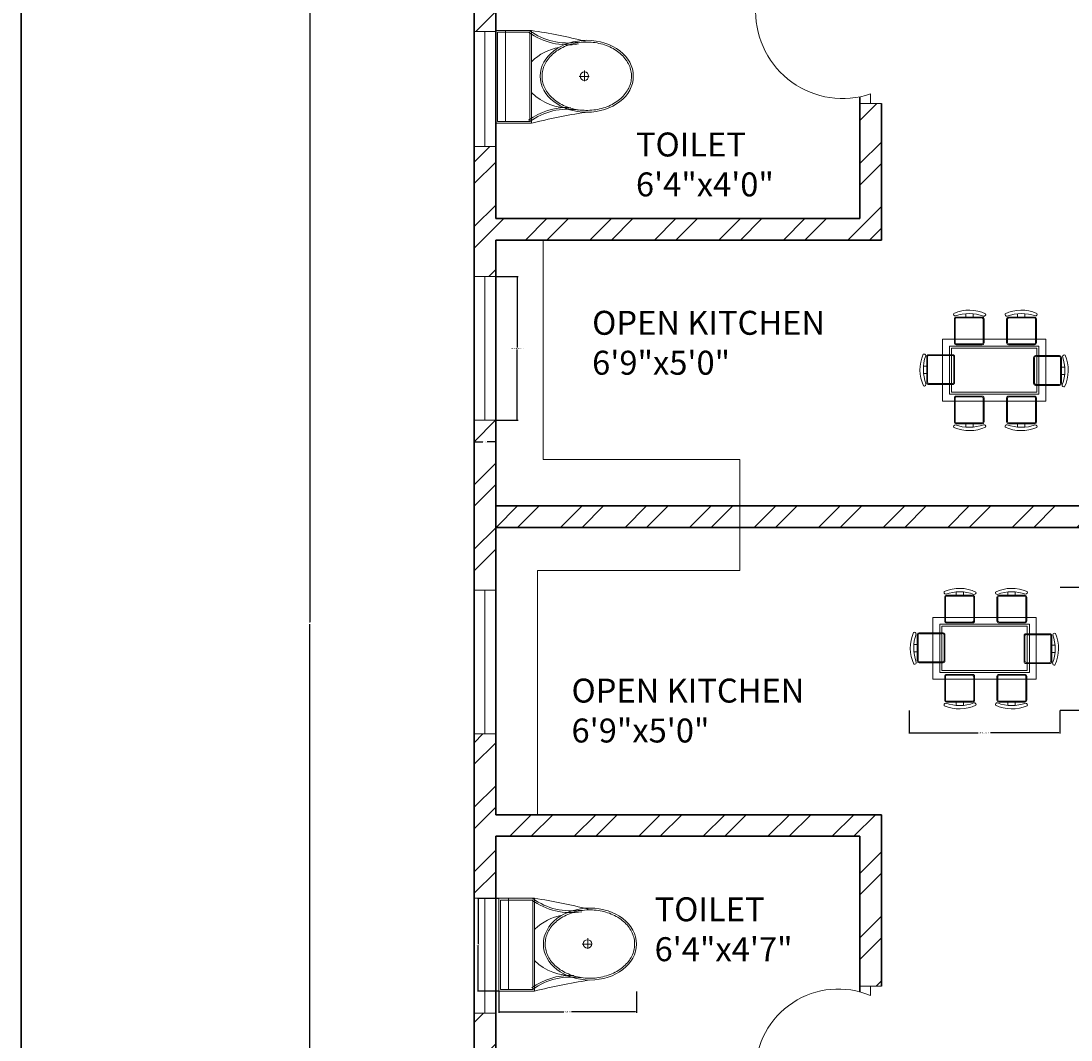
# Model space of a CAD drawing. Units: inches. Extents: x 2165 to 3042, y 1626 to 2968.
# Tile 2 of 11: x 2192 to 2411, y 1996 to 2208. Entities that reach past the tile are written whole.
import ezdxf

# ---------------------------------------------------------------- set-up
doc = ezdxf.new("R2010")
doc.units = ezdxf.units.IN
for name, color, linetype, lineweight in [('A-ANNO-DIMS', 2, 'Continuous', 18), ('A-AREA-IDEN', 7, 'Continuous', 18), ('A-DOOR', 3, 'Continuous', 18), ('A-FLOR-CASE', 8, 'Continuous', 18), ('A-FLOR-FIXT', 9, 'Continuous', 18), ('A-FURN', 8, 'Continuous', 13), ('A-GLAZ', 4, 'Continuous', 18), ('A-WALL', 7, 'Continuous', 35), ('A-WALL-PATT', 252, 'Continuous', 13)]:
    doc.layers.add(name, color=color, linetype=linetype, lineweight=lineweight)
doc.styles.get("Standard").update_dxf_attribs({"font": 'arial.ttf'})
doc.dimstyles.get("Standard").update_dxf_attribs({"dimtxt": 0.18, "dimasz": 0.18, "dimexe": 0.18, "dimexo": 0.0625, "dimgap": 0.09, "dimtad": 0, "dimtih": 1, "dimtoh": 1, "dimdec": 4, "dimzin": 0, "dimdsep": 46, "dimtxsty": 'Standard', "dimcen": 0.09, "dimadec": 0, "dimazin": 0, "dimtfac": 1, "dimtdec": 4, "dimtofl": 0, "dimtmove": 0, "dimatfit": 3, "dimfxl": 1, "dimtolj": 1, "dimtzin": 0, "dimarcsym": 0})

# ---------------------------------------------------------------- blocks, each defined once
blk = doc.blocks.new('A$C31115884')
for p, q in [((283.1, 497.7), (223.4, 497.7)), ((257.5, 466.4), (257.5, 523.2)), ((0, 200), (0, 0)), ((520, 200), (0, 200)), ((10, 190), (10, 10)), ((510, 190), (10, 190)), ((510, 10), (510, 190)), ((520, 0), (520, 200)), ((510, 54.5), (0, 54.5)), ((10, 10), (510, 10)), ((0, 0), (520, 0))]:
    blk.add_line(p, q)
blk.add_circle((255.6, 496.4), 23.6)
for centre, radius, start, end in [((2777.7, -204.6), 2807, 165.4549, 171.71327), ((3237, 905), 2807, 188.28673, 194.5451), ((-294.5, 403.3), 364.7, 324.20913, 9.34987), ((-294.5, 403.3), 374.7, 324.20913, 9.34987), ((139.5, 406.2), 293.5, 315.84364, 2.65635), ((805.8, 403.3), 364.7, 170.65013, 215.79087), ((383.6, 406.2), 293.5, 190.27735, 224.15636), ((805.8, 403.3), 374.7, 179.20365, 215.79087)]:
    blk.add_arc(centre, radius, start, end)
blk.add_ellipse((256.2, 509.9), major_axis=(0, -260.7), ratio=0.772727)
blk.add_open_spline([(256.2, 259.2), (263.1, 259.2), (270, 259.7), (287.8, 262.3), (298.7, 265.1), (319.9, 273.1), (330.2, 278.4), (350.1, 291.1), (359.7, 298.7), (377.7, 315.9), (386.2, 325.5), (401.7, 346.6), (408.8, 358.1), (421.3, 382.5), (426.8, 395.5), (435.9, 422.4), (439.5, 436.4), (444.8, 465.1), (446.5, 479.7), (447.9, 509.2), (447.6, 524), (445, 553.3), (442.7, 567.8), (436.3, 596), (432.1, 609.7), (421.9, 636), (416, 648.6), (402.5, 672.1), (395, 683), (378.6, 703), (369.8, 712.1), (351.1, 728), (341.3, 734.8), (320.9, 746.2), (310.4, 750.7), (288.9, 757.3), (278, 759.4), (256, 761), (245, 760.6), (223.1, 757.2), (212.3, 754.3), (191.1, 746.1), (180.8, 740.7), (160.9, 727.8), (151.4, 720.1), (133.5, 702.7), (125.1, 693), (109.6, 671.7), (102.6, 660.2), (90.2, 635.7), (84.9, 622.7), (76, 595.6), (72.4, 581.6), (67.2, 552.9), (65.6, 538.2), (64.4, 508.8), (64.8, 494), (67.5, 464.7), (69.9, 450.2), (76.6, 422), (80.8, 408.3), (91.1, 382.2), (97.2, 369.7), (110.8, 346.3), (118.4, 335.4), (134.8, 315.6), (143.7, 306.7), (162.4, 290.9), (172.3, 284.2), (192.8, 273), (203.3, 268.6), (224.8, 262.2), (235.8, 260.2), (249.9, 259.3), (253, 259.2), (256.2, 259.2)], degree=3, knots=[0, 0, 0, 0, 0.110105, 0.110105, 0.285049, 0.285049, 0.459994, 0.459994, 0.634938, 0.634938, 0.809882, 0.809882, 0.984827, 0.984827, 1.159771, 1.159771, 1.334715, 1.334715, 1.50966, 1.50966, 1.684604, 1.684604, 1.859549, 1.859549, 2.034493, 2.034493, 2.209437, 2.209437, 2.384382, 2.384382, 2.559326, 2.559326, 2.73427, 2.73427, 2.909215, 2.909215, 3.084159, 3.084159, 3.259103, 3.259103, 3.434048, 3.434048, 3.608992, 3.608992, 3.783936, 3.783936, 3.958881, 3.958881, 4.133825, 4.133825, 4.30877, 4.30877, 4.483714, 4.483714, 4.658658, 4.658658, 4.833603, 4.833603, 5.008547, 5.008547, 5.183491, 5.183491, 5.358436, 5.358436, 5.53338, 5.53338, 5.708324, 5.708324, 5.883269, 5.883269, 6.058213, 6.058213, 6.233158, 6.233158, 6.283185, 6.283185, 6.283185, 6.283185])
blk = doc.blocks.new('DINING-SET-6-SEAT')
for points in [[(7.39, 23.96, -0.175809), (13.27, 23.92, 0.578392), (13.71, 24.41, 0.214524), (7.08, 24.5, 0.552014), (7.39, 23.96, -0.065079)], [(7.39, 23.96, -0.175809), (13.27, 23.92, 0.578392), (13.71, 24.41, 0.214524), (7.08, 24.5, 0.552014), (7.39, 23.96, -0.065079)], [(11.1, 23.73), (11.1, 24.42, -0.064759)], [(11.1, 23.73), (11.1, 24.42, -0.064759)], [(18.21, 23.92, -0.578392), (17.77, 24.41, -0.214524), (24.4, 24.5, -0.552014), (24.09, 23.96, 0.175809), (18.21, 23.92)], [(18.21, 23.92, -0.578392), (17.77, 24.41, -0.214524), (24.4, 24.5, -0.552014), (24.09, 23.96, 0.175809), (18.21, 23.92)], [(20.38, 23.73), (20.38, 24.42, 0.064759)], [(20.38, 23.73), (20.38, 24.42, 0.064759)], [(13.02, 23.73), (7.56, 23.73, 0.414214), (7.18, 23.35), (7.18, 18.33, 0.414214), (7.56, 17.95), (13.02, 17.95, 0.414214), (13.4, 18.33), (13.4, 23.35, 0.414214), (13.02, 23.73)], [(13.02, 23.73), (7.56, 23.73, 0.414214), (7.18, 23.35), (7.18, 18.33, 0.414214), (7.56, 17.95), (13.02, 17.95, 0.414214), (13.4, 18.33), (13.4, 23.35, 0.414214), (13.02, 23.73)], [(23.91, 23.73, -0.414214), (24.3, 23.35), (24.3, 18.33, -0.414214), (23.91, 17.95), (18.46, 17.95, -0.414214), (18.08, 18.33), (18.08, 23.35, -0.414214), (18.46, 23.73), (23.91, 23.73)], [(23.91, 23.73, -0.414214), (24.3, 23.35), (24.3, 18.33, -0.414214), (23.91, 17.95), (18.46, 17.95, -0.414214), (18.08, 18.33), (18.08, 23.35, -0.414214), (18.46, 23.73), (23.91, 23.73)], [(1.25, 9.78, -0.578392), (0.76, 9.33, -0.214524), (0.67, 15.96, -0.552014), (1.2, 15.65, 0.175809), (1.25, 9.78)], [(1.25, 9.78, -0.578392), (0.76, 9.33, -0.214524), (0.67, 15.96, -0.552014), (1.2, 15.65, 0.175809), (1.25, 9.78)], [(1.44, 15.48, -0.414214), (1.82, 15.86), (6.83, 15.86, -0.414214), (7.21, 15.48), (7.21, 10.03, -0.414214), (6.83, 9.65), (1.82, 9.65, -0.414214), (1.44, 10.03), (1.44, 15.48)], [(1.44, 15.48, -0.414214), (1.82, 15.86), (6.83, 15.86, -0.414214), (7.21, 15.48), (7.21, 10.03, -0.414214), (6.83, 9.64), (1.82, 9.64, -0.414214), (1.44, 10.03), (1.44, 15.48)], [(29.52, 15.29, 0.414214), (29.14, 15.68), (24.12, 15.68, 0.414214), (23.74, 15.29), (23.74, 9.84, 0.414214), (24.12, 9.46), (29.14, 9.46, 0.414214), (29.52, 9.84), (29.52, 15.29)], [(29.52, 15.29, 0.414214), (29.14, 15.67), (24.12, 15.67, 0.414214), (23.74, 15.29), (23.74, 9.84, 0.414214), (24.12, 9.46), (29.14, 9.46, 0.414214), (29.52, 9.84), (29.52, 15.29)], [(29.76, 15.47, -0.175809), (29.71, 9.59, 0.578392), (30.2, 9.15, 0.214524), (30.29, 15.78, 0.552014), (29.76, 15.47, -0.065079)], [(29.76, 15.47, -0.175809), (29.71, 9.59, 0.578392), (30.2, 9.15, 0.214524), (30.29, 15.78, 0.552014), (29.76, 15.47, -0.065079)], [(1.44, 11.94), (0.75, 11.94, 0.064759)], [(1.44, 11.94), (0.75, 11.94, 0.064759)], [(29.52, 11.76), (30.21, 11.76, -0.064759)], [(29.52, 11.76), (30.21, 11.76, -0.064759)], [(13.02, 1.44), (7.56, 1.44, -0.414214), (7.18, 1.82), (7.18, 6.83, -0.414214), (7.56, 7.21), (13.02, 7.21, -0.414214), (13.4, 6.83), (13.4, 1.82, -0.414214), (13.02, 1.44)], [(13.02, 1.44), (7.56, 1.44, -0.414214), (7.18, 1.82), (7.18, 6.83, -0.414214), (7.56, 7.21), (13.02, 7.21, -0.414214), (13.4, 6.83), (13.4, 1.82, -0.414214), (13.02, 1.44)], [(23.91, 1.44, 0.414214), (24.3, 1.82), (24.3, 6.83, 0.414214), (23.91, 7.21), (18.46, 7.21, 0.414214), (18.08, 6.83), (18.08, 1.82, 0.414214), (18.46, 1.44), (23.91, 1.44)], [(23.91, 1.44, 0.414214), (24.3, 1.82), (24.3, 6.83, 0.414214), (23.91, 7.21), (18.46, 7.21, 0.414214), (18.08, 6.83), (18.08, 1.82, 0.414214), (18.46, 1.44), (23.91, 1.44)], [(13.27, 1.25, -0.578392), (13.71, 0.76, -0.214524), (7.08, 0.67, -0.552014), (7.39, 1.2, 0.175809), (13.27, 1.25)], [(13.27, 1.25, -0.578392), (13.71, 0.76, -0.214524), (7.08, 0.67, -0.552014), (7.39, 1.2, 0.175809), (13.27, 1.25)], [(11.1, 1.44), (11.1, 0.75, 0.064759)], [(11.1, 1.44), (11.1, 0.75, 0.064759)], [(24.09, 1.2, -0.175809), (18.21, 1.25, 0.578392), (17.77, 0.76, 0.214524), (24.4, 0.67, 0.552014), (24.09, 1.2, -0.065079)], [(24.09, 1.2, -0.175809), (18.21, 1.25, 0.578392), (17.77, 0.76, 0.214524), (24.4, 0.67, 0.552014), (24.09, 1.2, -0.065079)], [(20.38, 1.44), (20.38, 0.75, -0.064759)], [(20.38, 1.44), (20.38, 0.75, -0.064759)]]:
    blk.add_lwpolyline(points, format="xyb")
for points in [[(9.57, 24.43), (9.57, 23.73)], [(9.57, 24.43), (9.57, 23.73)], [(21.9, 24.43), (21.9, 23.73)], [(21.9, 24.43), (21.9, 23.73)], [(0.73, 13.47), (1.44, 13.47)], [(0.73, 13.47), (1.44, 13.47)], [(30.22, 13.28), (29.52, 13.28)], [(30.22, 13.28), (29.52, 13.28)], [(9.57, 0.73), (9.57, 1.44)], [(9.57, 0.73), (9.57, 1.44)], [(21.9, 0.73), (21.9, 1.44)], [(21.9, 0.73), (21.9, 1.44)]]:
    blk.add_lwpolyline(points)
for points in [[(7.57, 23.56), (12.84, 23.56, -0.414214), (13.23, 23.17), (13.23, 18.5, -0.414214), (12.84, 18.12), (7.57, 18.12, -0.512069), (7.35, 18.5), (7.35, 23.17, -0.512069)], [(7.57, 23.56), (12.84, 23.56, -0.414214), (13.23, 23.17), (13.23, 18.5, -0.414214), (12.84, 18.12), (7.57, 18.12, -0.512069), (7.35, 18.5), (7.35, 23.17, -0.512069)], [(23.91, 23.56), (18.63, 23.56, 0.414214), (18.25, 23.17), (18.25, 18.5, 0.414214), (18.63, 18.12), (23.91, 18.12, 0.512069), (24.12, 18.5), (24.12, 23.17, 0.512069)], [(23.91, 23.56), (18.63, 23.56, 0.414214), (18.25, 23.17), (18.25, 18.5, 0.414214), (18.63, 18.12), (23.91, 18.12, 0.512069), (24.12, 18.5), (24.12, 23.17, 0.512069)], [(1.61, 15.48), (1.61, 10.2, 0.414214), (1.99, 9.82), (6.66, 9.82, 0.414214), (7.04, 10.2), (7.04, 15.48, 0.512069), (6.66, 15.69), (1.99, 15.69, 0.512069)], [(1.61, 15.48), (1.61, 10.2, 0.414214), (1.99, 9.82), (6.66, 9.82, 0.414214), (7.04, 10.2), (7.04, 15.48, 0.512069), (6.66, 15.69), (1.99, 15.69, 0.512069)], [(29.35, 15.29), (29.35, 10.01, -0.414214), (28.97, 9.63), (24.3, 9.63, -0.414214), (23.92, 10.01), (23.92, 15.29, -0.512069), (24.3, 15.5), (28.97, 15.5, -0.512069)], [(29.35, 15.29), (29.35, 10.01, -0.414214), (28.97, 9.63), (24.3, 9.63, -0.414214), (23.92, 10.01), (23.92, 15.29, -0.512069), (24.3, 15.5), (28.97, 15.5, -0.512069)], [(7.57, 1.61), (12.84, 1.61, 0.414214), (13.23, 1.99), (13.23, 6.66, 0.414214), (12.84, 7.04), (7.57, 7.04, 0.512069), (7.35, 6.66), (7.35, 1.99, 0.512069)], [(7.57, 1.61), (12.84, 1.61, 0.414214), (13.23, 1.99), (13.23, 6.66, 0.414214), (12.84, 7.04), (7.57, 7.04, 0.512069), (7.35, 6.66), (7.35, 1.99, 0.512069)], [(23.91, 1.61), (18.63, 1.61, -0.414214), (18.25, 1.99), (18.25, 6.66, -0.414214), (18.63, 7.04), (23.91, 7.04, -0.512069), (24.12, 6.66), (24.12, 1.99, -0.512069)], [(23.91, 1.61), (18.63, 1.61, -0.414214), (18.25, 1.99), (18.25, 6.66, -0.414214), (18.63, 7.04), (23.91, 7.04, -0.512069), (24.12, 6.66), (24.12, 1.99, -0.512069)]]:
    blk.add_lwpolyline(points, format="xyb", close=True)
for points in [[(4.72, 19.12), (26.29, 19.12), (26.29, 6.18), (4.72, 6.18)], [(4.72, 19.12), (26.29, 19.12), (26.29, 6.18), (4.72, 6.18)], [(6.16, 17.68), (24.85, 17.68), (24.85, 7.62), (6.16, 7.62)], [(6.16, 17.68), (24.85, 17.68), (24.85, 7.62), (6.16, 7.62)], [(6.59, 17.25), (24.42, 17.25), (24.42, 8.05), (6.59, 8.05)], [(6.59, 17.25), (24.42, 17.25), (24.42, 8.05), (6.59, 8.05)]]:
    blk.add_lwpolyline(points, close=True)
blk = doc.blocks.new('WIN-24')
for p, q in [((0, 0), (0, 4.5)), ((0, 4.5), (0, 2.25)), ((24, 2.25), (24, 4.5)), ((24, 4.5), (24, 0)), ((0, 2.25), (24, 2.25))]:
    blk.add_line(p, q)
blk = doc.blocks.new('WIN-30')
for p, q in [((4.5, 30), (0, 30)), ((0, 30), (2.25, 30)), ((2.25, 30), (2.25, 0)), ((2.25, 0), (0, 0)), ((0, 0), (4.5, 0))]:
    blk.add_line(p, q)
blk = doc.blocks.new('*D20')
at = {"layer": 'A-ANNO-DIMS', "color": 0, "lineweight": -2, "transparency": 16777216}
for p, q in [((2291.76, 2005.69), (2291.76, 2001.26)), ((2320.48, 2005.69), (2320.48, 2001.26)), ((2291.94, 2001.44), (2305.34, 2001.44)), ((2320.3, 2001.44), (2306.89, 2001.44))]:
    blk.add_line(p, q, dxfattribs=at)
at = {"layer": 'A-ANNO-DIMS', "color": 0, "transparency": 16777216}
for points in [[(2291.94, 2001.47), (2291.94, 2001.41), (2291.76, 2001.44)], [(2320.3, 2001.47), (2320.3, 2001.41), (2320.48, 2001.44)]]:
    blk.add_solid(points, dxfattribs=at)
at = {"layer": 'Defpoints', "color": 0, "transparency": 16777216}
for p in [(2291.76, 2005.75), (2320.48, 2005.75), (2320.48, 2001.44)]:
    blk.add_point(p, dxfattribs=at)
at = {"layer": 'A-ANNO-DIMS', "color": 0, "transparency": 16777216, "insert": (2306.12, 2001.44), "char_height": 0.18, "attachment_point": 5}
blk.add_mtext('\\A1;WC 29 TYP.', dxfattribs=at)
blk = doc.blocks.new('*D21')
at = {"layer": 'A-ANNO-DIMS', "color": 0, "lineweight": -2, "transparency": 16777216}
for p, q in [((2291.7, 2025.13), (2287.27, 2025.13)), ((2287.45, 2024.95), (2287.45, 2015.62)), ((2287.45, 2005.93), (2287.45, 2015.26)), ((2291.7, 2005.75), (2287.27, 2005.75))]:
    blk.add_line(p, q, dxfattribs=at)
at = {"layer": 'A-ANNO-DIMS', "color": 0, "transparency": 16777216}
for points in [[(2287.42, 2024.95), (2287.48, 2024.95), (2287.45, 2025.13)], [(2287.42, 2005.93), (2287.48, 2005.93), (2287.45, 2005.75)]]:
    blk.add_solid(points, dxfattribs=at)
at = {"layer": 'Defpoints', "color": 0, "transparency": 16777216}
for p in [(2291.76, 2025.13), (2287.45, 2005.75), (2291.76, 2005.75)]:
    blk.add_point(p, dxfattribs=at)
at = {"layer": 'A-ANNO-DIMS', "color": 0, "transparency": 16777216, "insert": (2287.45, 2015.44), "char_height": 0.18, "attachment_point": 5}
blk.add_mtext('\\A1;19 TYP.', dxfattribs=at)
blk = doc.blocks.new('*D30')
at = {"layer": 'A-ANNO-DIMS', "color": 0, "lineweight": -2, "transparency": 16777216}
for p, q in [((2377.4, 2064.36), (2377.4, 2059.52)), ((2408.86, 2064.36), (2408.86, 2059.52)), ((2377.58, 2059.7), (2391.85, 2059.7)), ((2408.68, 2059.7), (2394.41, 2059.7))]:
    blk.add_line(p, q, dxfattribs=at)
at = {"layer": 'A-ANNO-DIMS', "color": 0, "transparency": 16777216}
for points in [[(2377.58, 2059.73), (2377.58, 2059.67), (2377.4, 2059.7)], [(2408.68, 2059.73), (2408.68, 2059.67), (2408.86, 2059.7)]]:
    blk.add_solid(points, dxfattribs=at)
at = {"layer": 'Defpoints', "color": 0, "transparency": 16777216}
for p in [(2377.4, 2064.42), (2408.86, 2064.42), (2408.86, 2059.7)]:
    blk.add_point(p, dxfattribs=at)
at = {"layer": 'A-ANNO-DIMS', "color": 0, "transparency": 16777216, "insert": (2393.13, 2059.7), "char_height": 0.18, "attachment_point": 5}
blk.add_mtext('\\A1;DINING SET 31 TYP.', dxfattribs=at)
blk = doc.blocks.new('*D31')
at = {"layer": 'A-ANNO-DIMS', "color": 0, "lineweight": -2, "transparency": 16777216}
for p, q in [((2408.92, 2090.09), (2413.76, 2090.09)), ((2413.58, 2089.91), (2413.58, 2077.44)), ((2413.58, 2064.6), (2413.58, 2077.08)), ((2408.92, 2064.42), (2413.76, 2064.42))]:
    blk.add_line(p, q, dxfattribs=at)
at = {"layer": 'A-ANNO-DIMS', "color": 0, "transparency": 16777216}
for points in [[(2413.55, 2089.91), (2413.61, 2089.91), (2413.58, 2090.09)], [(2413.55, 2064.6), (2413.61, 2064.6), (2413.58, 2064.42)]]:
    blk.add_solid(points, dxfattribs=at)
at = {"layer": 'Defpoints', "color": 0, "transparency": 16777216}
for p in [(2408.86, 2090.09), (2413.58, 2090.09), (2408.86, 2064.42)]:
    blk.add_point(p, dxfattribs=at)
at = {"layer": 'A-ANNO-DIMS', "color": 0, "transparency": 16777216, "insert": (2413.58, 2077.26), "char_height": 0.18, "attachment_point": 5}
blk.add_mtext('\\A1;26 TYP.', dxfattribs=at)
blk = doc.blocks.new('*D38')
at = {"layer": 'A-ANNO-DIMS', "color": 0, "lineweight": -2, "transparency": 16777216}
for p, q in [((2291.17, 2154.94), (2295.78, 2154.94)), ((2295.6, 2154.76), (2295.6, 2140.12)), ((2295.6, 2125.12), (2295.6, 2139.75)), ((2291.17, 2124.94), (2295.78, 2124.94))]:
    blk.add_line(p, q, dxfattribs=at)
at = {"layer": 'A-ANNO-DIMS', "color": 0, "transparency": 16777216}
for points in [[(2295.57, 2154.76), (2295.63, 2154.76), (2295.6, 2154.94)], [(2295.57, 2125.12), (2295.63, 2125.12), (2295.6, 2124.94)]]:
    blk.add_solid(points, dxfattribs=at)
at = {"layer": 'Defpoints', "color": 0, "transparency": 16777216}
for p in [(2291.1, 2154.94), (2295.6, 2154.94), (2291.1, 2124.94)]:
    blk.add_point(p, dxfattribs=at)
at = {"layer": 'A-ANNO-DIMS', "color": 0, "transparency": 16777216, "insert": (2295.6, 2139.94), "char_height": 0.18, "attachment_point": 5}
blk.add_mtext('\\A1;KITCHEN WINDOW 30 TYP.', dxfattribs=at)
blk = doc.blocks.new('*D39')
at = {"layer": 'A-ANNO-DIMS', "color": 0, "lineweight": -2, "transparency": 16777216}
for p, q in [((2286.6, 2124.88), (2286.6, 2120.26)), ((2291.1, 2124.88), (2291.1, 2120.26)), ((2286.78, 2120.44), (2288.4, 2120.44)), ((2290.92, 2120.44), (2289.31, 2120.44))]:
    blk.add_line(p, q, dxfattribs=at)
at = {"layer": 'A-ANNO-DIMS', "color": 0, "transparency": 16777216}
for points in [[(2286.78, 2120.47), (2286.78, 2120.41), (2286.6, 2120.44)], [(2290.92, 2120.47), (2290.92, 2120.41), (2291.1, 2120.44)]]:
    blk.add_solid(points, dxfattribs=at)
at = {"layer": 'Defpoints', "color": 0, "transparency": 16777216}
for p in [(2286.6, 2124.94), (2291.1, 2124.94), (2291.1, 2120.44)]:
    blk.add_point(p, dxfattribs=at)
at = {"layer": 'A-ANNO-DIMS', "color": 0, "transparency": 16777216, "insert": (2288.85, 2120.44), "char_height": 0.18, "attachment_point": 5}
blk.add_mtext('\\A1;5 TYP.', dxfattribs=at)
blk = doc.blocks.new('*D51')
at = {"layer": 'A-ANNO-DIMS', "color": 0, "lineweight": -2, "transparency": 16777216}
for p, q in [((2387.04, 2363.58), (2252.12, 2363.58)), ((2252.3, 2363.4), (2252.3, 2082.76)), ((2252.3, 1801.76), (2252.3, 2082.4)), ((2535.54, 1801.58), (2252.12, 1801.58))]:
    blk.add_line(p, q, dxfattribs=at)
at = {"layer": 'A-ANNO-DIMS', "color": 0, "transparency": 16777216}
for points in [[(2252.27, 2363.4), (2252.33, 2363.4), (2252.3, 2363.58)], [(2252.27, 1801.76), (2252.33, 1801.76), (2252.3, 1801.58)]]:
    blk.add_solid(points, dxfattribs=at)
at = {"layer": 'Defpoints', "color": 0, "transparency": 16777216}
for p in [(2252.3, 2363.58), (2387.1, 2363.58), (2535.6, 1801.58)]:
    blk.add_point(p, dxfattribs=at)
at = {"layer": 'A-ANNO-DIMS', "color": 0, "transparency": 16777216, "insert": (2252.3, 2082.58), "char_height": 0.18, "attachment_point": 5}
blk.add_mtext('\\A1;562', dxfattribs=at)

msp = doc.modelspace()

# ---------------------------------------------------------------- hatches: boundary and pattern name
at = {"layer": 'A-WALL-PATT'}
h = msp.add_hatch(dxfattribs=at)
h.set_pattern_fill('ANSI32', color=256)
h.paths.add_polyline_path([(2406.4931, 2332.0783), (2286.6045, 2332.0783), (2286.6045, 2310.967), (2288.8545, 2310.967), (2291.1045, 2310.967), (2291.1045, 2327.5783), (2406.4931, 2327.5783), (2406.4931, 2329.8283)])
h.paths.add_polyline_path([(2439.6045, 2327.5783), (2444.9584, 2327.5783), (2444.9584, 2332.0783), (2430.2901, 2332.0783), (2430.2901, 2329.8283), (2430.2901, 2327.5783), (2435.1045, 2327.5783), (2435.1045, 2219.5783), (2431.0902, 2219.5783), (2431.0902, 2215.0783), (2435.1045, 2215.0783), (2444.1108, 2215.0783), (2444.1108, 2217.3283), (2444.1108, 2219.5783), (2439.6045, 2219.5783)])
h.paths.add_polyline_path([(2497.5418, 2329.8283), (2497.5418, 2332.0783), (2470.1978, 2332.0783), (2470.1978, 2327.5783), (2497.5418, 2327.5783)])
h.paths.add_polyline_path([(2617.9543, 2332.0783), (2557.5418, 2332.0783), (2557.5418, 2327.5783), (2583.6045, 2327.5783), (2583.6045, 2219.5783), (2474.0523, 2219.5783), (2474.0523, 2215.0783), (2583.6045, 2215.0783), (2583.6045, 2107.0783), (2579.3609, 2107.0783), (2579.3609, 2102.5783), (2588.1045, 2102.5783), (2593.5283, 2102.5783), (2593.5283, 2104.8283), (2593.5283, 2107.0783), (2588.1045, 2107.0783), (2588.1045, 2215.0783), (2691.2325, 2215.0783), (2691.2325, 2217.3283), (2691.2325, 2219.5783), (2588.1045, 2219.5783), (2588.1045, 2327.5783), (2617.9543, 2327.5783)])
h.paths.add_polyline_path([(2702.4444, 2329.8283), (2702.4444, 2332.0783), (2677.9543, 2332.0783), (2677.9543, 2327.5783), (2702.4444, 2327.5783)])
h.paths.add_polyline_path([(2736.6045, 2327.5783), (2742.5161, 2327.5783), (2742.5161, 2329.8283), (2742.5161, 2332.0783), (2727.7639, 2332.0783), (2727.7639, 2329.8283), (2727.7639, 2327.5783), (2732.1045, 2327.5783), (2732.1045, 2219.5783), (2726.4404, 2219.5783), (2726.4404, 2215.0783), (2732.1045, 2215.0783), (2742.7291, 2215.0783), (2742.7291, 2217.3283), (2742.7291, 2219.5783), (2736.6045, 2219.5783)])
h.paths.add_polyline_path([(2885.1045, 2332.0783), (2768.4887, 2332.0783), (2768.4887, 2327.5783), (2784.6045, 2327.5783), (2880.6045, 2327.5783), (2880.6045, 2310.967), (2885.1045, 2310.967)])
h.paths.add_polyline_path([(2885.1045, 2250.967), (2880.6045, 2250.967), (2880.6045, 2219.5783), (2776.5755, 2219.5783), (2776.5755, 2215.0783), (2788.1045, 2215.0783), (2788.1045, 2209.8634), (2790.3545, 2209.8634), (2792.6045, 2209.8634), (2792.6045, 2215.0783), (2880.6045, 2215.0783), (2880.6045, 2139.0783), (2871.2037, 2139.0783), (2871.2037, 2134.5783), (2885.1045, 2134.5783)])
h.paths.add_polyline_path([(2545.013, 2107.0783), (2474.0523, 2107.0783), (2291.1045, 2107.0783), (2291.1045, 2102.5783), (2535.6045, 2102.5783), (2535.6045, 2096.8046), (2537.8545, 2096.8046), (2540.1045, 2096.8046), (2540.1045, 2102.5783), (2545.013, 2102.5783), (2545.013, 2104.8283)])
h.paths.add_polyline_path([(2397.7297, 2217.3283), (2397.7297, 2219.5783), (2291.1045, 2219.5783), (2291.1045, 2250.967), (2286.6045, 2250.967), (2286.6045, 2206.1346), (2288.8545, 2206.1346), (2291.1045, 2206.1346), (2291.1045, 2215.0783), (2367.1045, 2215.0783), (2367.1045, 2212.2868), (2371.6045, 2212.2868), (2371.6045, 2215.0783), (2397.7297, 2215.0783)])
h.paths.add_polyline_path([(2291.1045, 1978.5783), (2367.1045, 1978.5783), (2371.6045, 1978.5783), (2373.2641, 1978.5783), (2374.4883, 1978.5783), (2374.4883, 1980.8283), (2374.4883, 1983.0783), (2371.6045, 1983.0783), (2371.6045, 1986.964), (2369.9051, 1986.964), (2369.3545, 1986.964), (2367.1045, 1986.964), (2367.1045, 1983.0783), (2291.1045, 1983.0783), (2291.1045, 2001.1808), (2286.6045, 2001.1808), (2286.6045, 1947.0203), (2288.8545, 1947.0203), (2291.1045, 1947.0203)])
h.paths.add_polyline_path([(2291.1045, 1887.0203), (2286.6045, 1887.0203), (2286.6045, 1842.0783), (2381.2561, 1842.0783), (2381.2561, 1844.3283), (2381.2561, 1846.5783), (2363.1045, 1846.5783), (2291.1045, 1846.5783)])
h.paths.add_polyline_path([(2415.6045, 1978.5783), (2421.1681, 1978.5783), (2421.1681, 1983.0783), (2415.6045, 1983.0783), (2406.5227, 1983.0783), (2406.5227, 1980.8283), (2406.5227, 1978.5783), (2411.1045, 1978.5783), (2411.1045, 1846.5783), (2406.7549, 1846.5783), (2406.7549, 1842.0783), (2419.2885, 1842.0783), (2419.2885, 1844.3283), (2419.2885, 1846.5783), (2415.6045, 1846.5783)])
h.paths.add_polyline_path([(2586.6045, 1982.779), (2586.6045, 1991.5911), (2582.1045, 1991.5911), (2582.1045, 1982.779), (2540.1045, 1982.779), (2540.1045, 2036.779), (2582.1045, 2036.779), (2582.1045, 2027.6051), (2586.6045, 2027.6051), (2586.6045, 2041.279), (2582.1045, 2041.279), (2540.1045, 2041.279), (2540.1045, 2063.9064), (2537.8545, 2063.9064), (2535.6045, 2063.9064), (2535.6045, 1983.0783), (2455.068, 1983.0783), (2455.068, 1978.5783), (2535.6045, 1978.5783), (2535.6045, 1846.5783), (2522.622, 1846.5783), (2522.622, 1842.0783), (2535.6045, 1842.0783), (2535.6045, 1806.0783), (2535.6045, 1801.5783), (2556.726, 1801.5783), (2556.726, 1803.8283), (2556.726, 1806.0783), (2540.1045, 1806.0783), (2540.1045, 1842.0783), (2540.1045, 1846.5783), (2540.1045, 1978.279), (2586.6045, 1978.279)])
h.paths.add_polyline_path([(2636.1045, 1978.5783), (2717.6642, 1978.5783), (2717.6642, 1980.8283), (2717.6642, 1983.0783), (2636.1045, 1983.0783), (2636.1045, 2063.9064), (2633.8545, 2063.9064), (2631.6045, 2063.9064), (2631.6045, 1846.5783), (2631.6045, 1842.0783), (2631.6045, 1806.0783), (2604.726, 1806.0783), (2604.726, 1801.5783), (2636.1045, 1801.5783), (2636.1045, 1842.0783), (2644.3411, 1842.0783), (2644.3411, 1844.3283), (2644.3411, 1846.5783), (2636.1045, 1846.5783)])
h.paths.add_polyline_path([(2760.6045, 1978.5783), (2764.9931, 1978.5783), (2764.9931, 1983.0783), (2750.4727, 1983.0783), (2750.4727, 1980.8283), (2750.4727, 1978.5783), (2756.1045, 1978.5783), (2756.1045, 1846.5783), (2749.4543, 1846.5783), (2749.4543, 1842.0783), (2765.1894, 1842.0783), (2765.1894, 1846.5783), (2760.6045, 1846.5783)])
h.paths.add_polyline_path([(2880.6045, 1983.0783), (2804.6045, 1983.0783), (2804.6045, 1988.3825), (2802.3545, 1988.3825), (2800.1045, 1988.3825), (2800.1045, 1983.0783), (2800.1045, 1978.5783), (2880.6045, 1978.5783)])
h.paths.add_polyline_path([(2885.1045, 2075.5783), (2871.2037, 2075.5783), (2871.2037, 2071.0783), (2880.6045, 2071.0783), (2880.6045, 1948.8144), (2885.1045, 1948.8144)])
h.paths.add_polyline_path([(2885.1045, 1888.8144), (2880.6045, 1888.8144), (2880.6045, 1846.5783), (2792.1167, 1846.5783), (2792.1167, 1842.0783), (2885.1045, 1842.0783)])
h.paths.add_polyline_path([(2724.4848, 1846.5783), (2708.1045, 1846.5783), (2692.3411, 1846.5783), (2692.3411, 1842.0783), (2724.4848, 1842.0783), (2724.4848, 1844.3283)])
h.paths.add_polyline_path([(2474.622, 1844.4672), (2474.622, 1846.5783), (2444.7417, 1846.5783), (2444.7417, 1842.0783), (2474.622, 1842.0783)])
h = msp.add_hatch(dxfattribs=at)
h.set_pattern_fill('ANSI32', color=256)
h.paths.add_polyline_path([(2371.6045, 2191.0783), (2369.3545, 2191.0783), (2367.1045, 2191.0783), (2367.1045, 2167.0783), (2291.1045, 2167.0783), (2291.1045, 2182.1346), (2286.6045, 2182.1346), (2286.6045, 2154.9377), (2288.8545, 2154.9377), (2291.1045, 2154.9377), (2291.1045, 2162.5783), (2371.6045, 2162.5783)])
h.paths.add_polyline_path([(2291.1045, 2124.9377), (2286.6045, 2124.9377), (2286.6045, 2089.4443), (2288.8545, 2089.4443), (2291.1045, 2089.4443)])
h.paths.add_polyline_path([(2371.6045, 2042.5783), (2291.1045, 2042.5783), (2291.1045, 2059.4443), (2286.6045, 2059.4443), (2286.6045, 2025.1808), (2288.8545, 2025.1808), (2291.1045, 2025.1808), (2291.1045, 2038.0783), (2367.1045, 2038.0783), (2367.1045, 2006.8196), (2371.6045, 2006.8196)])

# ---------------------------------------------------------------- linework, layer by layer
at = {"layer": 'A-DOOR'}
for p, q in [((2369.3545, 2191.0783), (2369.3545, 2193.0783)), ((2367.1045, 2191.0783), (2371.6045, 2191.0783)), ((2371.6045, 2191.0783), (2369.3545, 2191.0783)), ((2367.1045, 2006.8196), (2371.6045, 2006.8196)), ((2371.6045, 2006.8196), (2369.3545, 2006.8196)), ((2369.3545, 2006.8196), (2369.3545, 2004.8196))]:
    msp.add_line(p, q, dxfattribs=at)
for centre, radius, start, end in [((2363.5239, 2210.2868), 18.1694, 180, 288.717485), ((2362.5919, 1988.964), 17.2375, 66.901381, 180)]:
    msp.add_arc(centre, radius, start, end, dxfattribs=at)
at = {"layer": 'A-FLOR-CASE'}
for p, q in [((2300.9892, 2162.5783), (2300.9892, 2162.5783)), ((2300.9892, 2162.5783), (2300.9892, 2116.7859)), ((2300.9892, 2116.7859), (2342.0306, 2116.7859)), ((2342.0306, 2116.7859), (2342.0306, 2107.0783)), ((2342.0306, 2107.0783), (2342.0306, 2093.5755)), ((2342.0306, 2093.5755), (2299.8015, 2093.5755)), ((2299.8015, 2093.5755), (2299.8015, 2042.5783))]:
    msp.add_line(p, q, dxfattribs=at)
at = {"layer": 'A-WALL'}
for p, q in [((2286.6045, 2332.0783), (2286.6045, 1842.0783)), ((2291.1045, 2215.0783), (2291.1045, 2167.0783)), ((2367.1045, 2192.4737), (2367.1045, 2167.0783)), ((2371.6045, 2191.0783), (2371.6045, 2162.5783)), ((2291.1045, 2167.0783), (2367.1045, 2167.0783)), ((2291.1045, 2162.5783), (2371.6045, 2162.5783)), ((2291.1045, 2162.5783), (2291.1045, 2042.5783)), ((2291.1045, 2107.0783), (2546.7118, 2107.0783)), ((2291.1045, 2102.5783), (2535.6045, 2102.5783)), ((2291.1045, 2042.5783), (2371.6045, 2042.5783)), ((2371.6045, 2006.8196), (2371.6045, 2042.5783)), ((2291.1045, 2038.0783), (2367.1045, 2038.0783)), ((2291.1045, 2038.0783), (2367.1045, 2038.0783)), ((2291.1045, 2038.0783), (2291.1045, 1983.0783)), ((2367.1045, 2038.0783), (2367.1045, 2005.6003))]:
    msp.add_line(p, q, dxfattribs=at)
msp.add_lwpolyline([(2191.9961, 2967.8547), (3042.3708, 2967.8547), (3042.3708, 1626.3264), (2191.9961, 1626.3264)], close=True, dxfattribs=at)

# ---------------------------------------------------------------- block references
at = {"layer": 'A-FLOR-FIXT', "xscale": 0.0372717239612423, "yscale": 0.0372717239612423, "zscale": 0.0372717239612423, "rotation": 270}
for p in [(2291.1045, 2206.3198), (2291.7576, 2025.1325)]:
    msp.add_blockref('A$C31115884', p, dxfattribs=at)
at = {"layer": 'A-FURN'}
for p in [(2379.661, 2122.769), (2377.6487, 2064.6772)]:
    msp.add_blockref('DINING-SET-6-SEAT', p, dxfattribs=at)
at = {"layer": 'A-GLAZ', "rotation": 90}
for p in [(2291.1048, 2182.135), (2291.1048, 2001.1811)]:
    msp.add_blockref('WIN-24', p, dxfattribs=at)
at = {"layer": 'A-GLAZ'}
for p in [(2286.604, 2124.9374), (2286.604, 2059.444)]:
    msp.add_blockref('WIN-30', p, dxfattribs=at)

# ---------------------------------------------------------------- texts
at = {"layer": 'A-AREA-IDEN', "char_height": 5, "attachment_point": 1}
for s, width, insert in [('TOILET\\P6\'4"x4\'0"', 80.665386, (2320.3721, 2185.0184)), ('OPEN KITCHEN\\P6\'9"x5\'0"', 75.850617, (2311.2303, 2147.7903)), ('OPEN KITCHEN\\P6\'9"x5\'0"', 128.511407, (2306.9228, 2071.0037)), ('TOILET\\P6\'4"x4\'7"', 105.52129, (2324.2687, 2025.3457))]:
    msp.add_mtext_dynamic_manual_height_columns(s, width=width, gutter_width=12.5, heights=[0], dxfattribs=dict(at, insert=insert))

# ---------------------------------------------------------------- dimensions: what is measured, and where the dimension line sits
at = {"layer": 'A-ANNO-DIMS'}
dim = msp.add_linear_dim(base=(2252.3045, 2363.5783), p1=(2535.6045, 1801.5783), p2=(2387.1045, 2363.5783), angle=90, dimstyle='Standard', override={"dimdec": 0, "dimlfac": 1, "dimrnd": 0, "dimzin": 0, "dimdsep": 46, "dimlunit": 2}, dxfattribs=at)
dim.commit()
dim.dimension.update_dxf_attribs({"geometry": '*D51', "text_midpoint": (2252.3045, 2082.5783)})
for base, p1, p2, angle, text, picture, middle in [((2295.6045, 2154.9377), (2291.1045, 2124.9377), (2291.1045, 2154.9377), 90, 'KITCHEN WINDOW <> TYP.', '*D38', (2295.6045, 2139.9377)), ((2413.579, 2090.0947), (2408.8594, 2064.4239), (2408.8594, 2090.0947), 90, '<> TYP.', '*D31', (2413.579, 2077.2593)), ((2287.4496, 2005.7512), (2291.7576, 2025.1325), (2291.7576, 2005.7512), 270, '<> TYP.', '*D21', (2287.4496, 2015.4419))]:
    dim = msp.add_linear_dim(base=base, p1=p1, p2=p2, angle=angle, text=text, dimstyle='Standard', override={"dimdec": 0, "dimlfac": 1, "dimrnd": 0, "dimzin": 0, "dimdsep": 46, "dimlunit": 2}, dxfattribs=at)
    dim.commit()
    dim.dimension.update_dxf_attribs({"geometry": picture, "text_midpoint": middle})
for base, p1, p2, text, picture, middle in [((2291.1044518572, 2120.4376971538), (2286.6044518572, 2124.9376971538), (2291.1044518572, 2124.9376971538), '<> TYP.', '*D39', (2288.8544518572, 2120.4376971538)), ((2408.8594, 2059.7043), (2377.3957, 2064.4239), (2408.8594, 2064.4239), 'DINING SET <> TYP.', '*D30', (2393.1276, 2059.7043)), ((2320.4781, 2001.4432), (2291.7576, 2005.7512), (2320.4781, 2005.7512), 'WC <> TYP.', '*D20', (2306.1179, 2001.4432))]:
    dim = msp.add_linear_dim(base=base, p1=p1, p2=p2, text=text, dimstyle='Standard', override={"dimdec": 0, "dimlfac": 1, "dimrnd": 0, "dimzin": 0, "dimdsep": 46, "dimlunit": 2}, dxfattribs=at)
    dim.commit()
    dim.dimension.update_dxf_attribs({"geometry": picture, "text_midpoint": middle})

doc.saveas('drawing.dxf')
